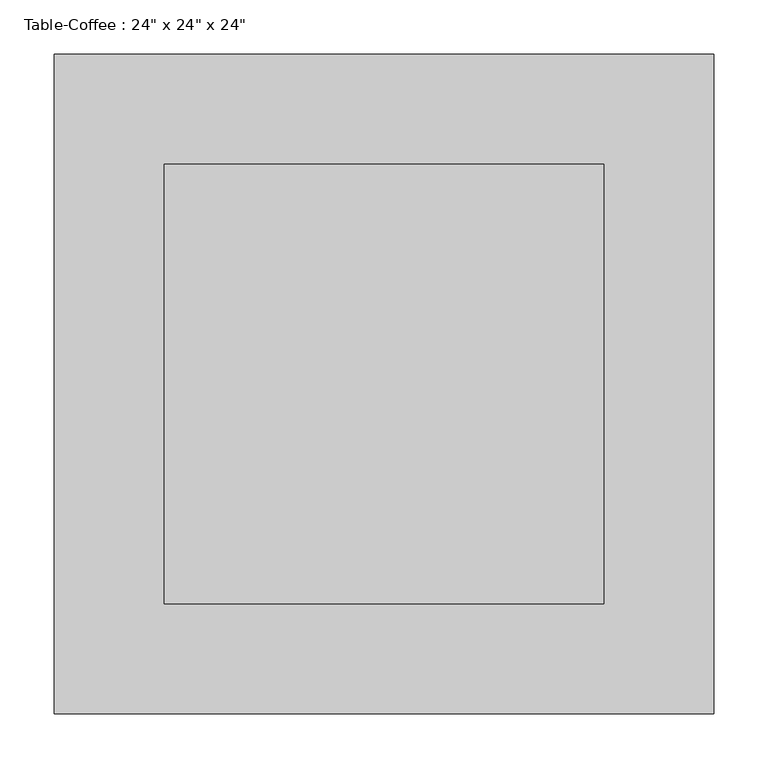
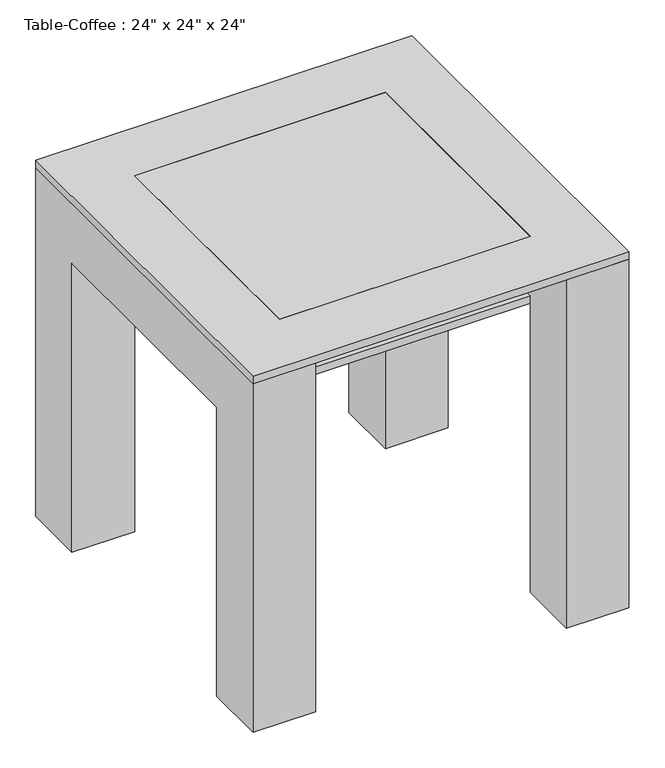
"""IFC4 building model written with IfcOpenShell, lengths in millimetres: furniture geometry."""

from ifc_helpers import new_model, si_unit, frame, origin, place, context, project, spatial, polyline, outline, extrude, source, transform, mapped, element, save


def furniture_d3665cec(model_context):
    return source(origin(), model_context, "Body", "SweptSolid", [
        extrude(outline(polyline([(323.0657667, 400.0110778), (323.0657667, -209.5889222), (-286.5342333, -209.5889222), (-286.5342333, 400.0110778), (323.0657667, 400.0110778)]), holes=[polyline([(221.4657667, 298.4110778), (-184.9342333, 298.4110778), (-184.9342333, -107.9889222), (221.4657667, -107.9889222), (221.4657667, 298.4110778)])]), frame((0.0, 0.0, 596.9), z_axis=(0.0, 0.0, 1.0), x_axis=(1.0, 0.0, 0.0)), (0.0, 0.0, 1.0), 12.7),
        extrude(outline(polyline([(221.4657667, 298.4110778), (221.4657667, -107.9889222), (-184.9342333, -107.9889222), (-184.9342333, 298.4110778), (221.4657667, 298.4110778)])), frame((0.0, 0.0, 596.9), z_axis=(0.0, 0.0, 1.0), x_axis=(1.0, 0.0, 0.0)), (0.0, 0.0, 1.0), 12.7),
        extrude(outline(polyline([(400.0110778, 596.9), (400.0110778, 0.0), (298.4110778, 0.0), (298.4110778, 495.3), (-107.9889222, 495.3), (-107.9889222, 0.0), (-209.5889222, 0.0), (-209.5889222, 596.9), (400.0110778, 596.9)])), frame((-286.5342333, 0.0, 0.0), z_axis=(1.0, 0.0, 0.0), x_axis=(0.0, 1.0, 0.0)), (0.0, 0.0, 1.0), 101.6),
        extrude(outline(polyline([(400.0110778, 0.0), (298.4110778, 0.0), (298.4110778, 495.3), (-107.9889222, 495.3), (-107.9889222, 0.0), (-209.5889222, 0.0), (-209.5889222, 596.9), (400.0110778, 596.9), (400.0110778, 0.0)])), frame((221.4657667, 0.0, 0.0), z_axis=(1.0, 0.0, 0.0), x_axis=(0.0, 1.0, 0.0)), (0.0, 0.0, 1.0), 101.6),
        extrude(outline(polyline([(221.4657667, 298.4110778), (221.4657667, -107.9889222), (-184.9342333, -107.9889222), (-184.9342333, 298.4110778), (221.4657667, 298.4110778)])), frame((0.0, 0.0, 495.3), z_axis=(0.0, 0.0, 1.0), x_axis=(1.0, 0.0, 0.0)), (0.0, 0.0, 1.0), 12.7),
    ])


if __name__ == "__main__":
    model = new_model("IFC4")
    model_context = context("Model", 3, world=origin())
    ifc_project = project(units=[si_unit("LENGTHUNIT", "METRE", prefix="MILLI")], contexts=[model_context])
    site = spatial("IfcSite", under=ifc_project)
    building = spatial("IfcBuilding", under=site)
    placement = place(None, origin())
    furniture_shape = furniture_d3665cec(model_context)
    element("IfcFurniture", 1, ObjectType="Table-Coffee : 24\" x 24\" x 24\"", at=placement, inside=building, context=model_context, shape_type="MappedRepresentation", body=[
        mapped(furniture_shape, transform((0.0, 0.0, 0.0), x_axis=(1.0, 0.0, 0.0), y_axis=(0.0, 1.0, 0.0), z_axis=(0.0, 0.0, 1.0))),
    ])
    save(model, "model.ifc")

# Revit data of these elements
# Type "Table-Coffee : 24\" x 24\" x 24\""
#   Assembly Code = "E2020200"
#   Height = 2' - 0"
#   Length = 2' - 0"
#   Width = 2' - 0"
#   Top Material = none
#   Frame Material = none
#   Default Elevation = 0
# Element 1 (IfcFurniture, "Table-Coffee : 24\" x 24\" x 24\"")
#   Materials on its faces: "Glass - Clear, Grey"
# Materials
#   "Glass - Clear, Grey": colour RGB 252 255 255, transparency 0.64
